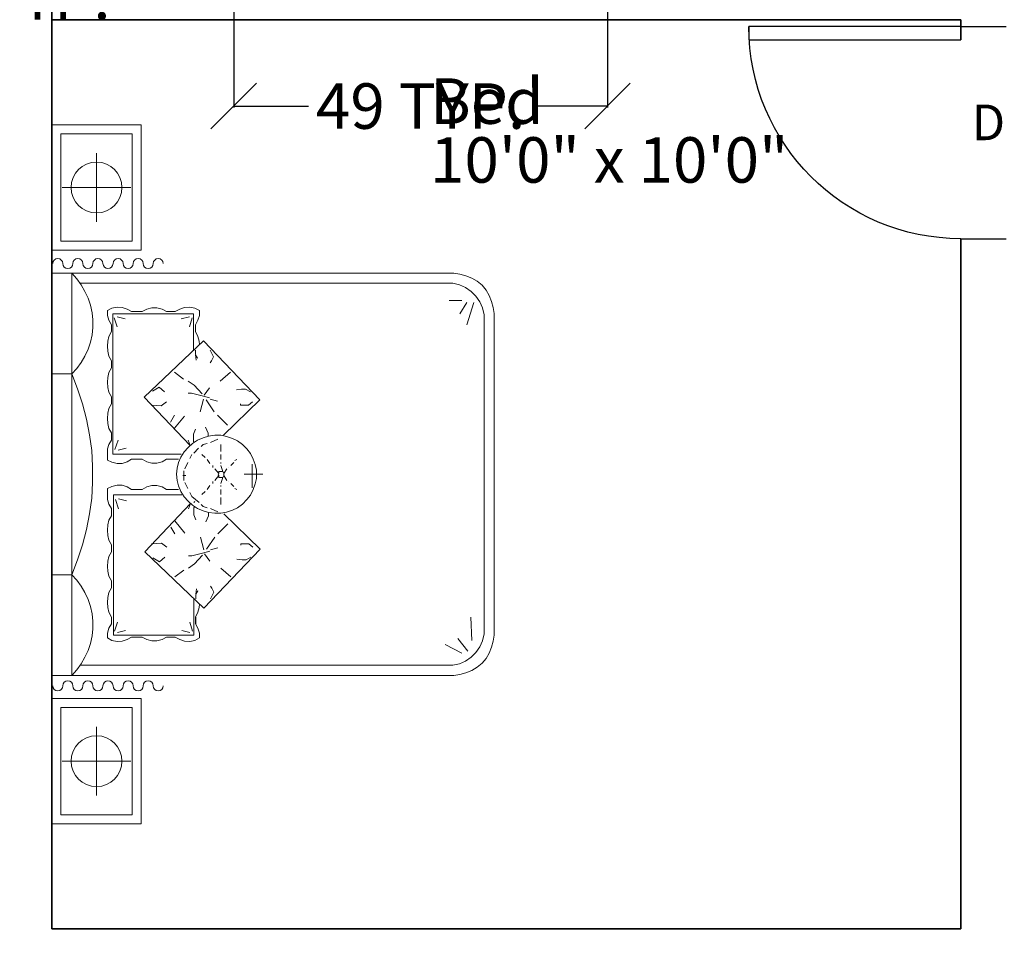
# Model space of a CAD drawing. Units: inches. Extents: x -1198 to -69, y -512 to 437.
# Tile 28 of 50: x -696 to -566, y 37 to 158. Entities that reach past the tile are written whole.
import ezdxf

# ---------------------------------------------------------------- set-up
doc = ezdxf.new("R2010")
doc.units = ezdxf.units.IN
doc.header["$MEASUREMENT"] = 0
for name, color, linetype, lineweight in [('A-ANNO-DIMS', 2, 'Continuous', 18), ('A-ANNO-SYMB', 7, 'Continuous', 18), ('A-AREA-IDEN', 7, 'Continuous', 18), ('A-FURN', 60, 'Continuous', 18), ('A-WALL', 7, 'Continuous', 35), ('Doors', 140, 'Continuous', 25), ('ds_furniture_Pen_No__7', 7, 'Continuous', 18)]:
    doc.layers.add(name, color=color, linetype=linetype, lineweight=lineweight)
doc.styles.get("Standard").update_dxf_attribs({"font": 'arial.ttf'})
doc.dimstyles.get("Standard").update_dxf_attribs({"dimtxt": 6, "dimasz": 6, "dimexe": 0.18, "dimexo": 0.0625, "dimgap": 0.09, "dimtad": 0, "dimtih": 1, "dimtoh": 1, "dimdec": 0, "dimzin": 0, "dimdsep": 46, "dimlunit": 4, "dimtxsty": 'Standard', "dimblk": 'OBLIQUE', "dimcen": 0.09, "dimadec": 0, "dimazin": 0, "dimtfac": 1, "dimtdec": 0, "dimtofl": 0, "dimtmove": 0, "dimatfit": 3, "dimfxl": 1, "dimtolj": 1, "dimtzin": 0, "dimarcsym": 0})

# ---------------------------------------------------------------- blocks, each defined once
blk = doc.blocks.new('*U4')
for p, q in [((0, 0), (0, -6)), ((28, 0), (28, -6))]:
    blk.add_line(p, q)
blk.add_lwpolyline([(0, 0), (0, 28), (1.75, 28), (1.75, 0)], close=True)
blk.add_arc((0, 0), 28, 0, 90)
blk = doc.blocks.new('new')
at = {"layer": 'ds_furniture_Pen_No__7'}
for p, q in [((-1180, 2274.4), (-1838.2, 2274.4)), ((-1838.2, 2274.4), (-1838.2, 1804.2)), ((-1180, 1804.2), (-1180, 2274.4)), ((-1057.8, 158.7), (-1057.8, 2274.4)), ((-1057.8, 2274.4), (1057.8, 2274.4)), ((-1057.8, 2274.4), (1057.8, 2274.4)), ((-1057.8, 158.7), (-1057.8, 2274.4)), ((-528.9, 2274.4), (-528.9, 2168.6)), ((528.9, 2274.4), (528.9, 2168.6)), ((1057.8, 2274.4), (1057.8, 158.7)), ((1057.8, 2274.4), (1057.8, 158.7)), ((1180, 1804.2), (1180, 2274.4)), ((1180, 2274.4), (1838.2, 2274.4)), ((1838.2, 2274.4), (1838.2, 1804.2)), ((-1227, 2227.4), (-1791.2, 2227.4)), ((-1791.2, 2227.4), (-1791.2, 1851.2)), ((-1509.1, 2220.2), (-1509.1, 1858.4)), ((-1227, 1851.2), (-1227, 2227.4)), ((1227, 1851.2), (1227, 2227.4)), ((1227, 2227.4), (1791.2, 2227.4)), ((1509.1, 2220.2), (1509.1, 1858.4)), ((1791.2, 2227.4), (1791.2, 1851.2)), ((1057.8, 2168.6), (-1057.8, 2168.6)), ((-1057.8, 2168.6), (-1028.2, 2143.2)), ((-1028.2, 2143.2), (-996.5, 2119.9)), ((-588.2, 2119.9), (-556.4, 2143.2)), ((-556.4, 2143.2), (-528.9, 2168.6)), ((-528.9, 2168.6), (-450.6, 2139)), ((-450.6, 2139), (-370.2, 2113.6)), ((370.2, 2113.6), (450.6, 2139)), ((450.6, 2139), (528.9, 2168.6)), ((528.9, 2168.6), (556.4, 2143.2)), ((556.4, 2143.2), (588.2, 2119.9)), ((996.5, 2119.9), (1028.2, 2143.2)), ((1028.2, 2143.2), (1057.8, 2168.6)), ((-1005, 165), (-1005, 2124.2)), ((-996.5, 2119.9), (-962.6, 2100.9)), ((-962.6, 2100.9), (-926.7, 2084)), ((-926.7, 2084), (-890.7, 2071.3)), ((-696.1, 2071.3), (-658, 2084)), ((-658, 2084), (-622, 2100.9)), ((-622, 2100.9), (-588.2, 2119.9)), ((-370.2, 2113.6), (-289.9, 2092.4)), ((-289.9, 2092.4), (-207.3, 2075.5)), ((-207.3, 2075.5), (-124.8, 2064.9)), ((124.8, 2064.9), (207.3, 2075.5)), ((207.3, 2075.5), (289.9, 2092.4)), ((289.9, 2092.4), (370.2, 2113.6)), ((588.2, 2119.9), (622, 2100.9)), ((622, 2100.9), (658, 2084)), ((658, 2084), (696.1, 2071.3)), ((890.7, 2071.3), (926.7, 2084)), ((926.7, 2084), (962.6, 2100.9)), ((962.6, 2100.9), (996.5, 2119.9)), ((1005, 2124.2), (1005, 165)), ((-1690.1, 2039.3), (-1328.2, 2039.3)), ((-890.7, 2071.3), (-850.5, 2062.8)), ((-850.5, 2062.8), (-812.4, 2058.6)), ((-812.4, 2058.6), (-772.2, 2058.6)), ((-772.2, 2058.6), (-734.1, 2062.8)), ((-734.1, 2062.8), (-696.1, 2071.3)), ((-124.8, 2064.9), (-42.3, 2060.7)), ((-42.3, 2060.7), (42.3, 2060.7)), ((42.3, 2060.7), (124.8, 2064.9)), ((696.1, 2071.3), (734.1, 2062.8)), ((734.1, 2062.8), (772.2, 2058.6)), ((772.2, 2058.6), (812.4, 2058.6)), ((812.4, 2058.6), (850.5, 2062.8)), ((850.5, 2062.8), (890.7, 2071.3)), ((1690.1, 2039.3), (1328.2, 2039.3)), ((-873.8, 1959.1), (-861.1, 1982.4)), ((-861.1, 1982.4), (-835.7, 1982.4)), ((-835.7, 1982.4), (-810.3, 1973.9)), ((-810.3, 1973.9), (-787, 1961.2)), ((-751.1, 1961.2), (-725.7, 1973.9)), ((-725.7, 1973.9), (-700.3, 1980.3)), ((-700.3, 1980.3), (-674.9, 1982.4)), ((-674.9, 1982.4), (-647.4, 1980.3)), ((-647.4, 1980.3), (-622, 1973.9)), ((-622, 1973.9), (-596.6, 1961.2)), ((-560.7, 1961.2), (-535.3, 1973.9)), ((-535.3, 1973.9), (-509.9, 1980.3)), ((-509.9, 1980.3), (-484.5, 1982.4)), ((-484.5, 1982.4), (-457, 1980.3)), ((-457, 1980.3), (-431.6, 1973.9)), ((-431.6, 1973.9), (-408.3, 1961.2)), ((-370.2, 1961.2), (-347, 1973.9)), ((-347, 1973.9), (-321.6, 1980.3)), ((-321.6, 1980.3), (-294.1, 1982.4)), ((-294.1, 1982.4), (-266.6, 1980.3)), ((-266.6, 1980.3), (-241.2, 1973.9)), ((-241.2, 1973.9), (-217.9, 1961.2)), ((-179.8, 1961.2), (-156.6, 1973.9)), ((-156.6, 1973.9), (-133.3, 1982.4)), ((-133.3, 1982.4), (-105.8, 1982.4)), ((-105.8, 1982.4), (-74, 1982.4)), ((-74, 1982.4), (-63.5, 1959.1)), ((74, 1982.4), (63.5, 1959.1)), ((105.8, 1982.4), (74, 1982.4)), ((133.3, 1982.4), (105.8, 1982.4)), ((156.6, 1973.9), (133.3, 1982.4)), ((179.8, 1961.2), (156.6, 1973.9)), ((241.2, 1973.9), (217.9, 1961.2)), ((266.6, 1980.3), (241.2, 1973.9)), ((294.1, 1982.4), (266.6, 1980.3)), ((321.6, 1980.3), (294.1, 1982.4)), ((347, 1973.9), (321.6, 1980.3)), ((370.2, 1961.2), (347, 1973.9)), ((431.6, 1973.9), (408.3, 1961.2)), ((457, 1980.3), (431.6, 1973.9)), ((484.5, 1982.4), (457, 1980.3)), ((509.9, 1980.3), (484.5, 1982.4)), ((535.3, 1973.9), (509.9, 1980.3)), ((560.7, 1961.2), (535.3, 1973.9)), ((622, 1973.9), (596.6, 1961.2)), ((647.4, 1980.3), (622, 1973.9)), ((674.9, 1982.4), (647.4, 1980.3)), ((700.3, 1980.3), (674.9, 1982.4)), ((725.7, 1973.9), (700.3, 1980.3)), ((751.1, 1961.2), (725.7, 1973.9)), ((810.3, 1973.9), (787, 1961.2)), ((835.7, 1982.4), (810.3, 1973.9)), ((861.1, 1982.4), (835.7, 1982.4)), ((873.8, 1959.1), (861.1, 1982.4)), ((-880.1, 1931.6), (-873.8, 1959.1)), ((-878, 1904.1), (-880.1, 1931.6)), ((-846.3, 1527.5), (-846.3, 1950.7)), ((-846.3, 1950.7), (-107.9, 1950.7)), ((-831.5, 1929.5), (-820.9, 1887.2)), ((-825.1, 1944.3), (-778.6, 1929.5)), ((-787, 1961.2), (-751.1, 1961.2)), ((-596.6, 1961.2), (-560.7, 1961.2)), ((-408.3, 1961.2), (-370.2, 1961.2)), ((-217.9, 1961.2), (-179.8, 1961.2)), ((-133.3, 1940.1), (-181.9, 1923.2)), ((-129.1, 1923.2), (-139.6, 1880.9)), ((-107.9, 1950.7), (-107.9, 1591)), ((-63.5, 1959.1), (-57.1, 1931.6)), ((-57.1, 1931.6), (-57.1, 1904.1)), ((63.5, 1959.1), (57.1, 1931.6)), ((57.1, 1931.6), (57.1, 1904.1)), ((844.2, 1952.8), (105.8, 1952.8)), ((105.8, 1952.8), (105.8, 1593.1)), ((126.9, 1925.3), (137.5, 1883)), ((131.2, 1942.2), (179.8, 1925.3)), ((217.9, 1961.2), (179.8, 1961.2)), ((408.3, 1961.2), (370.2, 1961.2)), ((596.6, 1961.2), (560.7, 1961.2)), ((787, 1961.2), (751.1, 1961.2)), ((823, 1946.4), (776.5, 1931.6)), ((829.4, 1931.6), (818.8, 1889.3)), ((844.2, 1529.6), (844.2, 1952.8)), ((880.1, 1931.6), (873.8, 1959.1)), ((878, 1904.1), (880.1, 1931.6)), ((-869.6, 1878.7), (-878, 1904.1)), ((-856.9, 1855.5), (-869.6, 1878.7)), ((-65.6, 1878.7), (-80.4, 1855.5)), ((-57.1, 1904.1), (-65.6, 1878.7)), ((57.1, 1904.1), (65.6, 1878.7)), ((65.6, 1878.7), (80.4, 1855.5)), ((856.9, 1855.5), (869.6, 1878.7)), ((869.6, 1878.7), (878, 1904.1)), ((-1791.2, 1851.2), (-1227, 1851.2)), ((-856.9, 1798.3), (-856.9, 1855.5)), ((-80.4, 1855.5), (-80.4, 1798.3)), ((80.4, 1855.5), (80.4, 1798.3)), ((856.9, 1798.3), (856.9, 1855.5)), ((1791.2, 1851.2), (1227, 1851.2)), ((-1838.2, 1804.2), (-1180, 1804.2)), ((-875.9, 1747.6), (-869.6, 1775.1)), ((-869.6, 1775.1), (-856.9, 1798.3)), ((-704.5, 1474.6), (-408.3, 1785.6)), ((-408.3, 1785.6), (-154.4, 1544.5)), ((-80.4, 1798.3), (-65.6, 1775.1)), ((-65.6, 1775.1), (-59.2, 1747.6)), ((65.6, 1775.1), (59.2, 1747.6)), ((80.4, 1798.3), (65.6, 1775.1)), ((406.2, 1787.8), (152.3, 1546.6)), ((702.4, 1476.8), (406.2, 1787.8)), ((869.6, 1775.1), (856.9, 1798.3)), ((875.9, 1747.6), (869.6, 1775.1)), ((1838.2, 1804.2), (1180, 1804.2)), ((-875.9, 1722.2), (-875.9, 1747.6)), ((-869.6, 1694.7), (-875.9, 1722.2)), ((-440.1, 1743.3), (-461.2, 1707.4)), ((-366, 1749.7), (-361.8, 1696.8)), ((-59.2, 1722.2), (-65.6, 1694.7)), ((-59.2, 1747.6), (-59.2, 1722.2)), ((59.2, 1747.6), (59.2, 1722.2)), ((59.2, 1722.2), (65.6, 1694.7)), ((363.9, 1751.8), (359.7, 1698.9)), ((437.9, 1745.4), (459.1, 1709.5)), ((869.6, 1694.7), (875.9, 1722.2)), ((875.9, 1722.2), (875.9, 1747.6)), ((-856.9, 1671.4), (-869.6, 1694.7)), ((-856.9, 1624.9), (-856.9, 1671.4)), ((-461.2, 1707.4), (-435.8, 1679.9)), ((-361.8, 1696.8), (-382.9, 1669.3)), ((-65.6, 1694.7), (-80.4, 1671.4)), ((-80.4, 1671.4), (-80.4, 1607.9)), ((65.6, 1694.7), (80.4, 1671.4)), ((80.4, 1671.4), (80.4, 1607.9)), ((359.7, 1698.9), (380.8, 1671.4)), ((459.1, 1709.5), (433.7, 1682)), ((856.9, 1671.4), (869.6, 1694.7)), ((856.9, 1624.9), (856.9, 1671.4)), ((-869.6, 1601.6), (-856.9, 1624.9)), ((-539.5, 1627), (-503.5, 1580.4)), ((-277.2, 1648.1), (-313.1, 1627)), ((-245.4, 1627), (-308.9, 1574.1)), ((-91, 1595.2), (-61.4, 1607.9)), ((-61.4, 1607.9), (-31.7, 1614.3)), ((-31.7, 1614.3), (0, 1618.5)), ((0, 1618.5), (31.7, 1614.3)), ((31.7, 1614.3), (61.4, 1607.9)), ((61.4, 1607.9), (91, 1595.2)), ((243.3, 1629.1), (306.8, 1576.2)), ((275, 1650.2), (311, 1629.1)), ((537.4, 1629.1), (501.4, 1582.5)), ((869.6, 1601.6), (856.9, 1624.9)), ((-880.1, 1548.7), (-878, 1576.2)), ((-878, 1576.2), (-869.6, 1601.6)), ((-831.5, 1548.7), (-820.9, 1591)), ((-471.8, 1523.3), (-493, 1555)), ((-429.5, 1538.1), (-429.5, 1555)), ((-181.9, 1555), (-154.4, 1544.5)), ((-162.9, 1533.9), (-141.8, 1557.2)), ((-141.8, 1557.2), (-118.5, 1578.3)), ((-118.5, 1578.3), (-91, 1595.2)), ((-42.3, 1574.1), (-74, 1559.3)), ((-31.7, 1580.4), (-2.1, 1580.4)), ((19, 1580.4), (-10.6, 1580.4)), ((-6.3, 1584.7), (-6.3, 1569.8)), ((-6.3, 1584.7), (-6.3, 1569.8)), ((29.6, 1574.1), (61.4, 1559.3)), ((91, 1595.2), (118.5, 1578.3)), ((118.5, 1578.3), (141.8, 1557.2)), ((141.8, 1557.2), (162.9, 1533.9)), ((179.8, 1557.2), (152.3, 1546.6)), ((427.4, 1540.2), (427.4, 1557.2)), ((469.7, 1525.4), (490.8, 1557.2)), ((829.4, 1550.8), (818.8, 1593.1)), ((878, 1576.2), (869.6, 1601.6)), ((880.1, 1548.7), (878, 1576.2)), ((-873.8, 1521.2), (-880.1, 1548.7)), ((-861.1, 1497.9), (-873.8, 1521.2)), ((-651.6, 1527.5), (-846.3, 1527.5)), ((-810.3, 1506.4), (-835.7, 1497.9)), ((-825.1, 1533.9), (-778.6, 1548.7)), ((-787, 1519.1), (-810.3, 1506.4)), ((-772.2, 1517), (-789.2, 1517)), ((-751.1, 1519.1), (-787, 1519.1)), ((-761.7, 1517), (-772.2, 1517)), ((-751.1, 1517), (-761.7, 1517)), ((-725.7, 1506.4), (-751.1, 1519.1)), ((-700.3, 1500), (-725.7, 1506.4)), ((-655.9, 1517), (-634.7, 1517)), ((-634.7, 1517), (-613.6, 1506.4)), ((-613.6, 1506.4), (-630.5, 1517)), ((-630.5, 1517), (-603, 1512.7)), ((-425.3, 1481), (-471.8, 1523.3)), ((-414.7, 1481), (-429.5, 1538.1)), ((-213.7, 1527.5), (-239.1, 1517)), ((-175.6, 1527.5), (-213.7, 1527.5)), ((-192.5, 1478.9), (-179.8, 1508.5)), ((-179.8, 1508.5), (-162.9, 1533.9)), ((-175.6, 1527.5), (-171.4, 1523.3)), ((-116.4, 1538.1), (-148.1, 1500)), ((-148.1, 1527.5), (-143.9, 1521.2)), ((-116.4, 1538.1), (-95.2, 1548.7)), ((103.7, 1538.1), (82.5, 1548.7)), ((112.1, 1527.5), (137.5, 1502.1)), ((162.9, 1533.9), (179.8, 1508.5)), ((173.5, 1529.6), (169.3, 1525.4)), ((173.5, 1529.6), (211.6, 1529.6)), ((179.8, 1508.5), (192.5, 1478.9)), ((211.6, 1529.6), (237, 1519.1)), ((412.6, 1483.1), (427.4, 1540.2)), ((423.1, 1483.1), (469.7, 1525.4)), ((628.4, 1519.1), (600.9, 1514.8)), ((632.6, 1519.1), (611.4, 1508.5)), ((611.4, 1508.5), (628.4, 1519.1)), ((653.7, 1519.1), (632.6, 1519.1)), ((649.5, 1529.6), (844.2, 1529.6)), ((700.3, 1500), (725.7, 1506.4)), ((725.7, 1506.4), (751.1, 1519.1)), ((749, 1519.1), (759.5, 1519.1)), ((751.1, 1519.1), (787, 1519.1)), ((759.5, 1519.1), (770.1, 1519.1)), ((770.1, 1519.1), (787, 1519.1)), ((823, 1536), (776.5, 1550.8)), ((787, 1519.1), (810.3, 1506.4)), ((810.3, 1506.4), (835.7, 1497.9)), ((861.1, 1497.9), (873.8, 1521.2)), ((873.8, 1521.2), (880.1, 1548.7)), ((-835.7, 1497.9), (-861.1, 1497.9)), ((-393.5, 1178.4), (-704.5, 1474.6)), ((-683.4, 1497.9), (-700.3, 1500)), ((-457, 1442.9), (-418.9, 1470.4)), ((-404.1, 1442.9), (-414.7, 1481)), ((-397.8, 1474.6), (-330, 1491.6)), ((-393.5, 1459.8), (-330, 1417.5)), ((-217.9, 1449.3), (-249.7, 1464.1)), ((-201, 1449.3), (-192.5, 1478.9)), ((-169.3, 1478.9), (-175.6, 1457.7)), ((-169.3, 1478.9), (-158.7, 1489.4)), ((-91, 1468.3), (-105.8, 1485.2)), ((-59.2, 1442.9), (-80.4, 1457.7)), ((57.1, 1442.9), (78.3, 1457.7)), ((88.9, 1468.3), (103.7, 1485.2)), ((156.6, 1478.9), (146, 1489.4)), ((156.6, 1478.9), (162.9, 1457.7)), ((192.5, 1478.9), (201, 1449.3)), ((215.8, 1451.4), (201, 1451.4)), ((215.8, 1451.4), (247.5, 1466.2)), ((395.6, 1476.8), (327.9, 1493.7)), ((391.4, 1461.9), (327.9, 1419.6)), ((391.4, 1180.6), (702.4, 1476.8)), ((402, 1445), (412.6, 1483.1)), ((454.9, 1445), (416.8, 1472.5)), ((683.4, 1497.9), (700.3, 1500)), ((835.7, 1497.9), (861.1, 1497.9)), ((-655.9, 1438.7), (-619.9, 1421.7)), ((-619.9, 1421.7), (-598.7, 1432.3)), ((-598.7, 1432.3), (-588.2, 1438.7)), ((-397.8, 1438.7), (-387.2, 1400.6)), ((-260.2, 1347.7), (-313.1, 1400.6)), ((-217.9, 1449.3), (-203.1, 1449.3)), ((-205.2, 1417.5), (-201, 1449.3)), ((-205.2, 1385.8), (-205.2, 1417.5)), ((-196.8, 1400.6), (-179.8, 1438.7)), ((-38.1, 1428.1), (-48.7, 1428.1)), ((-6.3, 1396.4), (-31.7, 1417.5)), ((4.2, 1396.4), (29.6, 1417.5)), ((36, 1428.1), (46.5, 1428.1)), ((184.1, 1400.6), (167.1, 1438.7)), ((201, 1449.3), (205.2, 1417.5)), ((205.2, 1417.5), (205.2, 1385.8)), ((258.1, 1349.8), (311, 1402.7)), ((395.6, 1440.8), (385.1, 1402.7)), ((596.6, 1434.4), (586, 1440.8)), ((617.8, 1423.9), (596.6, 1434.4)), ((653.7, 1440.8), (617.8, 1423.9)), ((-539.5, 1332.9), (-493, 1385.8)), ((-393.5, 1178.4), (-207.3, 1368.9)), ((-198.9, 1356.2), (-205.2, 1385.8)), ((-188.3, 1324.4), (-198.9, 1356.2)), ((-122.7, 1385.8), (-158.7, 1385.8)), ((-80.4, 1385.8), (-105.8, 1385.8)), ((-59.2, 1385.8), (-63.5, 1385.8)), ((-16.9, 1375.2), (-48.7, 1385.8)), ((-6.3, 1368.9), (-31.7, 1354)), ((-16.9, 1385.8), (-16.9, 1396.4)), ((-16.9, 1396.4), (-6.3, 1396.4)), ((-16.9, 1375.2), (-16.9, 1385.8)), ((-6.3, 1368.9), (-16.9, 1375.2)), ((-6.3, 1396.4), (-2.1, 1398.5)), ((-6.3, 1368.9), (-2.1, 1368.9)), ((4.2, 1396.4), (-2.1, 1398.5)), ((4.2, 1368.9), (-2.1, 1368.9)), ((14.8, 1396.4), (4.2, 1396.4)), ((4.2, 1368.9), (14.8, 1375.2)), ((4.2, 1368.9), (29.6, 1354)), ((14.8, 1385.8), (14.8, 1396.4)), ((14.8, 1375.2), (14.8, 1385.8)), ((14.8, 1375.2), (46.5, 1385.8)), ((57.1, 1385.8), (61.4, 1385.8)), ((78.3, 1385.8), (103.7, 1385.8)), ((120.6, 1385.8), (156.6, 1385.8)), ((198.9, 1356.2), (188.3, 1324.4)), ((205.2, 1385.8), (198.9, 1356.2)), ((391.4, 1180.6), (205.2, 1371)), ((537.4, 1335), (490.8, 1387.9)), ((-450.6, 1273.6), (-446.4, 1301.2)), ((-175.6, 1296.9), (-188.3, 1324.4)), ((-156.6, 1271.5), (-175.6, 1296.9)), ((-74, 1311.7), (-80.4, 1301.2)), ((-48.7, 1332.9), (-63.5, 1316)), ((-38.1, 1343.5), (-38, 1343.5)), ((36, 1343.5), (36, 1343.5)), ((46.5, 1332.9), (61.4, 1316)), ((71.9, 1311.7), (78.3, 1301.2)), ((175.6, 1296.9), (156.6, 1271.5)), ((188.3, 1324.4), (175.6, 1296.9)), ((448.5, 1275.8), (444.3, 1303.3)), ((-450.6, 1252.5), (-450.6, 1273.6)), ((-435.8, 1227.1), (-450.6, 1252.5)), ((-366, 1280), (-372.4, 1280)), ((-366, 1237.7), (-366, 1280)), ((-133.3, 1248.3), (-156.6, 1271.5)), ((-110, 1229.2), (-133.3, 1248.3)), ((0, 1163.6), (0, 1263.1)), ((133.3, 1248.3), (110, 1229.2)), ((156.6, 1271.5), (133.3, 1248.3)), ((363.9, 1239.8), (363.9, 1282.1)), ((363.9, 1282.1), (370.2, 1282.1)), ((433.7, 1229.2), (448.5, 1254.6)), ((448.5, 1254.6), (448.5, 1275.8)), ((-382.9, 1216.5), (-366, 1237.7)), ((-80.4, 1214.4), (-110, 1229.2)), ((-50.8, 1203.8), (-80.4, 1214.4)), ((52.9, 1220.8), (-71.9, 1220.8)), ((-21.2, 1197.5), (-50.8, 1203.8)), ((0, 1197.5), (-21.2, 1197.5)), ((21.2, 1197.5), (0, 1197.5)), ((50.8, 1203.8), (21.2, 1197.5)), ((80.4, 1214.4), (50.8, 1203.8)), ((110, 1229.2), (80.4, 1214.4)), ((380.8, 1218.6), (363.9, 1239.8)), ((-1053.6, 126.9), (-1057.8, 158.7)), ((-1053.6, 126.9), (-1057.8, 158.7)), ((-996.5, 129.1), (-1005, 165)), ((-941.5, 116.4), (-894.9, 205.2)), ((914, 116.4), (914, 184.1)), ((1005, 165), (996.5, 129.1)), ((1057.8, 158.7), (1053.6, 126.9)), ((1057.8, 158.7), (1053.6, 126.9)), ((-1045.2, 95.2), (-1053.6, 126.9)), ((-1045.2, 95.2), (-1053.6, 126.9)), ((-983.8, 97.3), (-996.5, 129.1)), ((-930.9, 84.6), (-863.2, 137.5)), ((903.4, 91), (844.2, 126.9)), ((996.5, 129.1), (983.8, 97.3)), ((1053.6, 126.9), (1045.2, 95.2)), ((1053.6, 126.9), (1045.2, 95.2)), ((-1032.5, 63.5), (-1045.2, 95.2)), ((-1032.5, 63.5), (-1045.2, 95.2)), ((-1015.5, 36), (-1032.5, 63.5)), ((-1015.5, 36), (-1032.5, 63.5)), ((-962.6, 67.7), (-983.8, 97.3)), ((-937.3, 42.3), (-962.6, 67.7)), ((-873.8, 63.5), (-751.1, 69.8)), ((903.4, 52.9), (787, 91)), ((962.6, 67.7), (937.3, 42.3)), ((983.8, 97.3), (962.6, 67.7)), ((1032.5, 63.5), (1015.5, 36)), ((1032.5, 63.5), (1015.5, 36)), ((1045.2, 95.2), (1032.5, 63.5)), ((1045.2, 95.2), (1032.5, 63.5)), ((-994.4, 10.6), (-1015.5, 36)), ((-994.4, 10.6), (-1015.5, 36)), ((-969, -10.6), (-994.4, 10.6)), ((-969, -10.6), (-994.4, 10.6)), ((-907.6, 21.2), (-937.3, 42.3)), ((-875.9, 8.5), (-907.6, 21.2)), ((-839.9, 0), (-875.9, 8.5)), ((839.9, 0), (-839.9, 0)), ((875.9, 8.5), (839.9, 0)), ((907.6, 21.2), (875.9, 8.5)), ((937.3, 42.3), (907.6, 21.2)), ((994.4, 10.6), (969, -10.6)), ((994.4, 10.6), (969, -10.6)), ((1015.5, 36), (994.4, 10.6)), ((1015.5, 36), (994.4, 10.6)), ((-941.5, -27.5), (-969, -10.6)), ((-941.5, -27.5), (-969, -10.6)), ((-909.7, -40.2), (-941.5, -27.5)), ((-909.7, -40.2), (-941.5, -27.5)), ((-878, -48.7), (-909.7, -40.2)), ((-878, -48.7), (-909.7, -40.2)), ((-846.3, -52.9), (-878, -48.7)), ((-846.3, -52.9), (-878, -48.7)), ((878, -48.7), (846.3, -52.9)), ((878, -48.7), (846.3, -52.9)), ((909.7, -40.2), (878, -48.7)), ((909.7, -40.2), (878, -48.7)), ((941.5, -27.5), (909.7, -40.2)), ((941.5, -27.5), (909.7, -40.2)), ((969, -10.6), (941.5, -27.5)), ((969, -10.6), (941.5, -27.5)), ((846.3, -52.9), (-846.3, -52.9)), ((846.3, -52.9), (-846.3, -52.9))]:
    blk.add_line(p, q, dxfattribs=at)
for centre in [(-1509.1, 2039.3), (1509.1, 2039.3)]:
    blk.add_circle(centre, 133.9, dxfattribs=at)
for centre, start, end in [((-1112.8, 2243.5), 90, 270), ((1108.7, 2243.5), 270, 90), ((-1112.8, 2190.6), 270, 90), ((1108.7, 2190.6), 90, 270), ((-1112.8, 2137.7), 90, 270), ((1108.7, 2137.7), 270, 90), ((-1112.8, 2084.8), 270, 90), ((-1112.8, 2084.8), 270, 90), ((1108.7, 2084.8), 90, 270), ((1108.7, 2084.8), 90, 270), ((-1112.8, 2031.9), 90, 270), ((1108.7, 2031.9), 270, 90), ((-1112.8, 1979), 270, 90), ((1108.7, 1979), 90, 270), ((-1112.8, 1926.1), 90, 270), ((1108.7, 1926.1), 270, 90), ((-1112.8, 1873.2), 270, 90), ((1108.7, 1873.2), 90, 270), ((-1112.8, 1820.3), 90, 270), ((1108.7, 1820.3), 270, 90), ((-1112.8, 1767.4), 270, 90), ((1108.7, 1767.4), 90, 270), ((-1112.8, 1714.6), 90, 270), ((1108.7, 1714.6), 270, 90)]:
    blk.add_arc(centre, 26.4, start, end, dxfattribs=at)
blk = doc.blocks.new('_Oblique')
at = {"color": 0, "linetype": 'ByBlock', "lineweight": -2}
blk.add_line((-0.5, -0.5), (0.5, 0.5), dxfattribs=at)
blk = doc.blocks.new('*D34')
at = {"layer": 'A-ANNO-DIMS', "color": 0, "lineweight": -2, "ltscale": 10, "transparency": 16777216}
for p, q in [((-757.75, 165.22), (-757.75, 161.07)), ((-730.88, 165.22), (-730.88, 161.07)), ((-757.75, 161.25), (-730.88, 161.25)), ((-730.88, 161.25), (-724.88, 161.25))]:
    blk.add_line(p, q, dxfattribs=at)
at = {"layer": 'DEFPOINTS', "color": 0, "ltscale": 10, "transparency": 16777216}
for p in [(-757.75, 165.28), (-730.88, 165.28), (-730.88, 161.25)]:
    blk.add_point(p, dxfattribs=at)
at = {"layer": 'A-ANNO-DIMS', "color": 0, "lineweight": -2, "ltscale": 10, "transparency": 16777216, "xscale": 6, "yscale": 6, "zscale": 6, "rotation": 180}
blk.add_blockref('_Oblique', (-757.75, 161.25), dxfattribs=at)
at = {"layer": 'A-ANNO-DIMS', "color": 0, "lineweight": -2, "ltscale": 10, "transparency": 16777216, "xscale": 6, "yscale": 6, "zscale": 6}
blk.add_blockref('_Oblique', (-730.88, 161.25), dxfattribs=at)
at = {"layer": 'A-ANNO-DIMS', "color": 0, "ltscale": 10, "transparency": 16777216, "insert": (-703.82, 161.25), "char_height": 6, "attachment_point": 5}
blk.add_mtext('\\A1;D1 27 TYP.', dxfattribs=at)
blk = doc.blocks.new('*D57')
at = {"layer": 'A-ANNO-DIMS', "color": 0, "lineweight": -2, "ltscale": 10, "transparency": 16777216}
for p, q in [((-667.75, 161.17), (-667.75, 146.65)), ((-618.4, 161.17), (-618.4, 146.65)), ((-667.75, 146.83), (-657.89, 146.83)), ((-618.4, 146.83), (-628.26, 146.83))]:
    blk.add_line(p, q, dxfattribs=at)
at = {"layer": 'DEFPOINTS', "color": 0, "ltscale": 10, "transparency": 16777216}
for p in [(-667.75, 161.23), (-618.4, 161.23), (-618.4, 146.83)]:
    blk.add_point(p, dxfattribs=at)
at = {"layer": 'A-ANNO-DIMS', "color": 0, "lineweight": -2, "ltscale": 10, "transparency": 16777216, "xscale": 6, "yscale": 6, "zscale": 6, "rotation": 180}
blk.add_blockref('_Oblique', (-667.75, 146.83), dxfattribs=at)
at = {"layer": 'A-ANNO-DIMS', "color": 0, "lineweight": -2, "ltscale": 10, "transparency": 16777216, "xscale": 6, "yscale": 6, "zscale": 6}
blk.add_blockref('_Oblique', (-618.4, 146.83), dxfattribs=at)
at = {"layer": 'A-ANNO-DIMS', "color": 0, "ltscale": 10, "transparency": 16777216, "insert": (-643.08, 146.83), "char_height": 6, "attachment_point": 5}
blk.add_mtext('\\A1;49 TYP.', dxfattribs=at)
blk = doc.blocks.new('*D76')
at = {"layer": 'A-ANNO-DIMS', "color": 0, "lineweight": -2, "ltscale": 10, "transparency": 16777216}
for p, q in [((-711.13, -38.21), (-711.13, 433.18)), ((-711.13, 433), (-697.75, 433)), ((-697.75, -38.21), (-697.75, 433.18)), ((-697.75, 433), (-691.75, 433))]:
    blk.add_line(p, q, dxfattribs=at)
at = {"layer": 'DEFPOINTS', "color": 0, "ltscale": 10, "transparency": 16777216}
for p in [(-697.75, 433), (-711.13, -38.27), (-697.75, -38.27)]:
    blk.add_point(p, dxfattribs=at)
at = {"layer": 'A-ANNO-DIMS', "color": 0, "lineweight": -2, "ltscale": 10, "transparency": 16777216, "xscale": 6, "yscale": 6, "zscale": 6, "rotation": 180}
blk.add_blockref('_Oblique', (-711.13, 433), dxfattribs=at)
at = {"layer": 'A-ANNO-DIMS', "color": 0, "lineweight": -2, "ltscale": 10, "transparency": 16777216, "xscale": 6, "yscale": 6, "zscale": 6}
blk.add_blockref('_Oblique', (-697.75, 433), dxfattribs=at)
at = {"layer": 'A-ANNO-DIMS', "color": 0, "ltscale": 10, "transparency": 16777216, "insert": (-681.81, 433), "char_height": 6, "attachment_point": 5}
blk.add_mtext('\\A1;13.38', dxfattribs=at)

msp = doc.modelspace()

# ---------------------------------------------------------------- linework, layer by layer
at = {"layer": 'A-WALL', "ltscale": 10}
for p, q in [((-691.7509, 257.2277), (-691.7509, 38.2277)), ((-571.7509, 158.2277), (-691.7509, 158.2277)), ((-691.7509, 158.2277), (-691.7509, 38.2277)), ((-571.7509, 158.2277), (-571.7509, 155.5722)), ((-571.7509, 129.3222), (-571.7509, 38.2277)), ((-571.7509, 38.2277), (-691.7509, 38.2277))]:
    msp.add_line(p, q, dxfattribs=at)

# ---------------------------------------------------------------- block references
at = {"layer": 'A-FURN', "xscale": 0.0250833463801972, "yscale": 0.0250833463801972, "zscale": 0.0250833463801972, "rotation": 90}
msp.add_blockref('new', (-634.702, 98.2277), dxfattribs=at)
at = {"layer": 'Doors', "xscale": -1, "rotation": 90}
msp.add_blockref('*U4', (-571.7509, 157.3222), dxfattribs=at)

# ---------------------------------------------------------------- texts
at = {"layer": 'A-ANNO-SYMB', "ltscale": 10}
msp.add_text('D', height=4.6996, dxfattribs=at).set_placement((-570.3184, 142.3277))
at = {"layer": 'A-AREA-IDEN', "ltscale": 10, "char_height": 6, "attachment_point": 1}
for s, insert in [('Bed', (-641.8292, 150.4825)), ('10\'0" x 10\'0"', (-641.8292, 142.7185))]:
    msp.add_mtext_dynamic_manual_height_columns(s, width=57.976527, gutter_width=30, heights=[0], dxfattribs=dict(at, insert=insert))

# ---------------------------------------------------------------- dimensions: what is measured, and where the dimension line sits
at = {"layer": 'A-ANNO-DIMS', "ltscale": 10}
dim = msp.add_linear_dim(base=(-697.7509, 433.0036), p1=(-711.1319, -38.2723), p2=(-697.7509, -38.2723), dimstyle='Standard', override={"dimdec": 2, "dimlfac": 1, "dimrnd": 0, "dimzin": 0, "dimdsep": 46, "dimlunit": 2}, dxfattribs=at)
dim.commit()
dim.dimension.update_dxf_attribs({"geometry": '*D76', "text_midpoint": (-681.8137, 433.0036)})
for base, p1, p2, text, picture, middle in [((-730.8812, 161.2489), (-757.7509, 165.2794), (-730.8812, 165.2794), 'D1 <> TYP.', '*D34', (-703.8157, 161.2489)), ((-618.4019, 146.8277), (-667.7509, 161.2277), (-618.4019, 161.2277), '<> TYP.', '*D57', (-643.0764, 146.8277))]:
    dim = msp.add_linear_dim(base=base, p1=p1, p2=p2, text=text, dimstyle='Standard', override={"dimdec": 0, "dimlfac": 1, "dimrnd": 0, "dimzin": 0, "dimdsep": 46, "dimlunit": 2}, dxfattribs=at)
    dim.commit()
    dim.dimension.update_dxf_attribs({"geometry": picture, "text_midpoint": middle})

doc.saveas('drawing.dxf')
